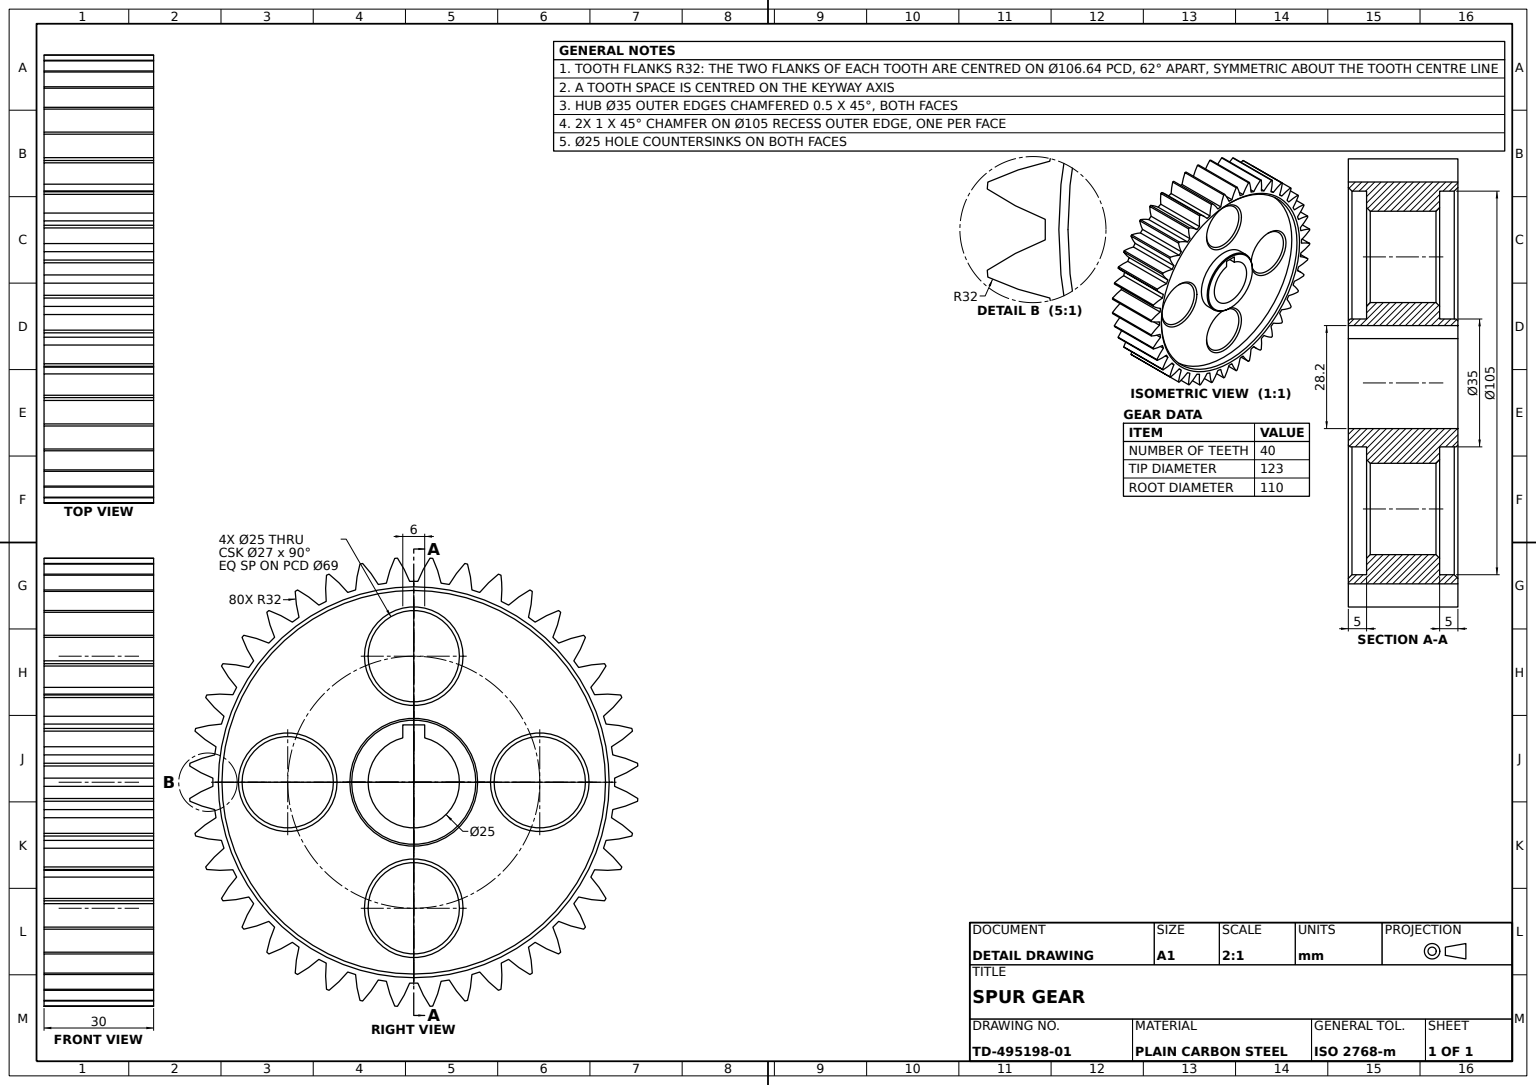
from build123d import *

# Parameters (mm, degrees)
GEAR_TOOTH_PROFILE_SKETCH_R       = 17.5
GEAR_BLANK_30MM_DEPTH             = 30
FRONT_RECESS_SKETCH_105_R         = 52.5
FRONT_WEB_RECESS_105X5_DEPTH      = 5
REAR_START                        = -5
REAR_RECESS_SKETCH_105_R          = 52.5
REAR_WEB_RECESS_105X5_DEPTH       = 5
REAR_RECESS_CHAMFER_1MM_SIZE      = 1
FRONT_RECESS_CHAMFER_1MM_SIZE     = 1
HUB_START                         = -20
HUB_SKETCH_35_R                   = 17.5
HUB_35_DEPTH                      = 20
KEYED_BORE_25_DEPTH               = 20
FRONT_START                       = 5
FRONT_HUB_BOSS_SKETCH_R           = 17.5
FRONT_HUB_BOSS_35X5_DEPTH         = 5
REAR_HUB_BOSS_SKETCH_R            = 17.5
REAR_HUB_BOSS_35X5_DEPTH          = 5
LIGHTENING_HOLES_SKETCH_4X_25_R   = 12.5
LIGHTENING_HOLES_4X_25_DEPTH      = 20
LIGHTENING_HOLE_CHAMFERS_1MM_SIZE = 1
FRONT_HUB_CHAMFER_0_5MM_SIZE      = 0.5
REAR_HUB_CHAMFER_0_5MM_SIZE       = 0.5


with BuildPart() as part:
    # Gear Tooth Profile Sketch → Gear Blank 30mm (new body)
    with BuildSketch(Plane.XY):
        with BuildLine():
            ThreePointArc((-13.990714351, 59.887477088), (-14.356889877, 59.800750104), (-14.722527887, 59.711784202))
            ThreePointArc((-14.722527887, 59.711784202), (-15.520987175, 56.212000648), (-15.922440287, 52.644808816))
            ThreePointArc((-15.922440287, 52.644808816), (-16.995934691, 52.308108396), (-18.062317448, 51.949520579))
            ThreePointArc((-18.062317448, 51.949520579), (-20.483842588, 54.599471175), (-23.186930882, 56.961532952))
            ThreePointArc((-23.186930882, 56.961532952), (-23.53503109, 56.818591249), (-23.882250156, 56.673522279))
            ThreePointArc((-23.882250156, 56.673522279), (-24.123392318, 53.091920316), (-23.961871129, 49.505845432))
            ThreePointArc((-23.961871129, 49.505845432), (-24.969477486, 49.00535883), (-25.966635809, 48.484366808))
            ThreePointArc((-25.966635809, 48.484366808), (-28.77289156, 50.722882124), (-31.812208221, 52.633006831))
            ThreePointArc((-31.812208221, 52.633006831), (-32.13366173, 52.437370108), (-32.453912166, 52.239770148))
            ThreePointArc((-32.453912166, 52.239770148), (-32.13179948, 48.664540704), (-31.41128118, 45.147883834))
            ThreePointArc((-31.41128118, 45.147883834), (-32.328188876, 44.495934691), (-33.231569417, 43.825367016))
            ThreePointArc((-33.231569417, 43.825367016), (-36.353456449, 45.597327377), (-39.654163416, 47.008481403))
            ThreePointArc((-39.654163416, 47.008481403), (-39.941054972, 46.764966884), (-40.22645115, 46.519701502))
            ThreePointArc((-40.22645115, 46.519701502), (-39.3490151, 43.038878591), (-38.08724124, 39.678231497))
            ThreePointArc((-38.08724124, 39.678231497), (-38.890872965, 38.890872965), (-39.678231497, 38.08724124))
            ThreePointArc((-39.678231497, 38.08724124), (-43.038878591, 39.3490151), (-46.519701502, 40.22645115))
            ThreePointArc((-46.519701502, 40.22645115), (-46.764966884, 39.941054972), (-47.008481403, 39.654163416))
            ThreePointArc((-47.008481403, 39.654163416), (-45.597327377, 36.353456449), (-43.825367016, 33.231569417))
            ThreePointArc((-43.825367016, 33.231569417), (-44.495934691, 32.328188876), (-45.147883834, 31.41128118))
            ThreePointArc((-45.147883834, 31.41128118), (-48.664540704, 32.13179948), (-52.239770148, 32.453912166))
            ThreePointArc((-52.239770148, 32.453912166), (-52.437370108, 32.13366173), (-52.633006831, 31.812208221))
            ThreePointArc((-52.633006831, 31.812208221), (-50.722882124, 28.77289156), (-48.484366808, 25.966635809))
            ThreePointArc((-48.484366808, 25.966635809), (-49.00535883, 24.969477486), (-49.505845432, 23.961871129))
            ThreePointArc((-49.505845432, 23.961871129), (-53.091920316, 24.123392318), (-56.673522279, 23.882250156))
            ThreePointArc((-56.673522279, 23.882250156), (-56.818591249, 23.53503109), (-56.961532952, 23.186930882))
            ThreePointArc((-56.961532952, 23.186930882), (-54.599471175, 20.483842588), (-51.949520579, 18.062317448))
            ThreePointArc((-51.949520579, 18.062317448), (-52.308108396, 16.995934691), (-52.644808816, 15.922440287))
            ThreePointArc((-52.644808816, 15.922440287), (-56.212000648, 15.520987175), (-59.711784202, 14.722527887))
            ThreePointArc((-59.711784202, 14.722527887), (-59.800750104, 14.356889877), (-59.887477088, 13.990714351))
            ThreePointArc((-59.887477088, 13.990714351), (-57.131640039, 11.690413431), (-54.135504743, 9.713244887))
            ThreePointArc((-54.135504743, 9.713244887), (-54.322858733, 8.603895577), (-54.487482289, 7.490946121))
            ThreePointArc((-54.487482289, 7.490946121), (-57.947954967, 6.536403817), (-61.279743827, 5.200288119))
            ThreePointArc((-61.279743827, 5.200288119), (-61.310416025, 4.825234387), (-61.338792782, 4.45))
            ThreePointArc((-61.338792782, 4.45), (-58.257038317, 2.609127496), (-54.988493114, 1.125))
            ThreePointArc((-54.988493114, 1.125), (-55, 0), (-54.988493114, -1.125))
            ThreePointArc((-54.988493114, -1.125), (-58.257038317, -2.609127496), (-61.338792782, -4.45))
            ThreePointArc((-61.338792782, -4.45), (-61.310416025, -4.825234387), (-61.279743827, -5.200288119))
            ThreePointArc((-61.279743827, -5.200288119), (-57.947954967, -6.536403817), (-54.487482289, -7.490946121))
            ThreePointArc((-54.487482289, -7.490946121), (-54.322858733, -8.603895577), (-54.135504743, -9.713244887))
            ThreePointArc((-54.135504743, -9.713244887), (-57.131640039, -11.690413431), (-59.887477088, -13.990714351))
            ThreePointArc((-59.887477088, -13.990714351), (-59.800750104, -14.356889877), (-59.711784202, -14.722527887))
            ThreePointArc((-59.711784202, -14.722527887), (-56.212000648, -15.520987175), (-52.644808816, -15.922440287))
            ThreePointArc((-52.644808816, -15.922440287), (-52.308108396, -16.995934691), (-51.949520579, -18.062317448))
            ThreePointArc((-51.949520579, -18.062317448), (-54.599471175, -20.483842588), (-56.961532952, -23.186930882))
            ThreePointArc((-56.961532952, -23.186930882), (-56.818591249, -23.53503109), (-56.673522279, -23.882250156))
            ThreePointArc((-56.673522279, -23.882250156), (-53.091920316, -24.123392318), (-49.505845432, -23.961871129))
            ThreePointArc((-49.505845432, -23.961871129), (-49.00535883, -24.969477486), (-48.484366808, -25.966635809))
            ThreePointArc((-48.484366808, -25.966635809), (-50.722882124, -28.77289156), (-52.633006831, -31.812208221))
            ThreePointArc((-52.633006831, -31.812208221), (-52.437370108, -32.13366173), (-52.239770148, -32.453912166))
            ThreePointArc((-52.239770148, -32.453912166), (-48.664540704, -32.13179948), (-45.147883834, -31.41128118))
            ThreePointArc((-45.147883834, -31.41128118), (-44.495934691, -32.328188876), (-43.825367016, -33.231569417))
            ThreePointArc((-43.825367016, -33.231569417), (-45.597327377, -36.353456449), (-47.008481403, -39.654163416))
            ThreePointArc((-47.008481403, -39.654163416), (-46.764966884, -39.941054972), (-46.519701502, -40.22645115))
            ThreePointArc((-46.519701502, -40.22645115), (-43.038878591, -39.3490151), (-39.678231497, -38.08724124))
            ThreePointArc((-39.678231497, -38.08724124), (-38.890872965, -38.890872965), (-38.08724124, -39.678231497))
            ThreePointArc((-38.08724124, -39.678231497), (-39.3490151, -43.038878591), (-40.22645115, -46.519701502))
            ThreePointArc((-40.22645115, -46.519701502), (-39.941054972, -46.764966884), (-39.654163416, -47.008481403))
            ThreePointArc((-39.654163416, -47.008481403), (-36.353456449, -45.597327377), (-33.231569417, -43.825367016))
            ThreePointArc((-33.231569417, -43.825367016), (-32.328188876, -44.495934691), (-31.41128118, -45.147883834))
            ThreePointArc((-31.41128118, -45.147883834), (-32.13179948, -48.664540704), (-32.453912166, -52.239770148))
            ThreePointArc((-32.453912166, -52.239770148), (-32.13366173, -52.437370108), (-31.812208221, -52.633006831))
            ThreePointArc((-31.812208221, -52.633006831), (-28.77289156, -50.722882124), (-25.966635809, -48.484366808))
            ThreePointArc((-25.966635809, -48.484366808), (-24.969477486, -49.00535883), (-23.961871129, -49.505845432))
            ThreePointArc((-23.961871129, -49.505845432), (-24.123392318, -53.091920316), (-23.882250156, -56.673522279))
            ThreePointArc((-23.882250156, -56.673522279), (-23.53503109, -56.818591249), (-23.186930882, -56.961532952))
            ThreePointArc((-23.186930882, -56.961532952), (-20.483842588, -54.599471175), (-18.062317448, -51.949520579))
            ThreePointArc((-18.062317448, -51.949520579), (-16.995934691, -52.308108396), (-15.922440287, -52.644808816))
            ThreePointArc((-15.922440287, -52.644808816), (-15.520987175, -56.212000648), (-14.722527887, -59.711784202))
            ThreePointArc((-14.722527887, -59.711784202), (-14.356889877, -59.800750104), (-13.990714351, -59.887477088))
            ThreePointArc((-13.990714351, -59.887477088), (-11.690413431, -57.131640039), (-9.713244887, -54.135504743))
            ThreePointArc((-9.713244887, -54.135504743), (-8.603895577, -54.322858733), (-7.490946121, -54.487482289))
            ThreePointArc((-7.490946121, -54.487482289), (-6.536403817, -57.947954967), (-5.200288119, -61.279743827))
            ThreePointArc((-5.200288119, -61.279743827), (-4.825234387, -61.310416025), (-4.45, -61.338792782))
            ThreePointArc((-4.45, -61.338792782), (-2.609127496, -58.257038317), (-1.125, -54.988493114))
            ThreePointArc((-1.125, -54.988493114), (0, -55), (1.125, -54.988493114))
            ThreePointArc((1.125, -54.988493114), (2.609127496, -58.257038317), (4.45, -61.338792782))
            ThreePointArc((4.45, -61.338792782), (4.825234387, -61.310416025), (5.200288119, -61.279743827))
            ThreePointArc((5.200288119, -61.279743827), (6.536403817, -57.947954967), (7.490946121, -54.487482289))
            ThreePointArc((7.490946121, -54.487482289), (8.603895577, -54.322858733), (9.713244887, -54.135504743))
            ThreePointArc((9.713244887, -54.135504743), (11.690413431, -57.131640039), (13.990714351, -59.887477088))
            ThreePointArc((13.990714351, -59.887477088), (14.356889877, -59.800750104), (14.722527887, -59.711784202))
            ThreePointArc((14.722527887, -59.711784202), (15.520987175, -56.212000648), (15.922440287, -52.644808816))
            ThreePointArc((15.922440287, -52.644808816), (16.995934691, -52.308108396), (18.062317448, -51.949520579))
            ThreePointArc((18.062317448, -51.949520579), (20.483842588, -54.599471175), (23.186930882, -56.961532952))
            ThreePointArc((23.186930882, -56.961532952), (23.53503109, -56.818591249), (23.882250156, -56.673522279))
            ThreePointArc((23.882250156, -56.673522279), (24.123392318, -53.091920316), (23.961871129, -49.505845432))
            ThreePointArc((23.961871129, -49.505845432), (24.969477486, -49.00535883), (25.966635809, -48.484366808))
            ThreePointArc((25.966635809, -48.484366808), (28.77289156, -50.722882124), (31.812208221, -52.633006831))
            ThreePointArc((31.812208221, -52.633006831), (32.13366173, -52.437370108), (32.453912166, -52.239770148))
            ThreePointArc((32.453912166, -52.239770148), (32.13179948, -48.664540704), (31.41128118, -45.147883834))
            ThreePointArc((31.41128118, -45.147883834), (32.328188876, -44.495934691), (33.231569417, -43.825367016))
            ThreePointArc((33.231569417, -43.825367016), (36.353456449, -45.597327377), (39.654163416, -47.008481403))
            ThreePointArc((39.654163416, -47.008481403), (39.941054972, -46.764966884), (40.22645115, -46.519701502))
            ThreePointArc((40.22645115, -46.519701502), (39.3490151, -43.038878591), (38.08724124, -39.678231497))
            ThreePointArc((38.08724124, -39.678231497), (38.890872965, -38.890872965), (39.678231497, -38.08724124))
            ThreePointArc((39.678231497, -38.08724124), (43.038878591, -39.3490151), (46.519701502, -40.22645115))
            ThreePointArc((46.519701502, -40.22645115), (46.764966884, -39.941054972), (47.008481403, -39.654163416))
            ThreePointArc((47.008481403, -39.654163416), (45.597327377, -36.353456449), (43.825367016, -33.231569417))
            ThreePointArc((43.825367016, -33.231569417), (44.495934691, -32.328188876), (45.147883834, -31.41128118))
            ThreePointArc((45.147883834, -31.41128118), (48.664540704, -32.13179948), (52.239770148, -32.453912166))
            ThreePointArc((52.239770148, -32.453912166), (52.437370108, -32.13366173), (52.633006831, -31.812208221))
            ThreePointArc((52.633006831, -31.812208221), (50.722882124, -28.77289156), (48.484366808, -25.966635809))
            ThreePointArc((48.484366808, -25.966635809), (49.00535883, -24.969477486), (49.505845432, -23.961871129))
            ThreePointArc((49.505845432, -23.961871129), (53.091920316, -24.123392318), (56.673522279, -23.882250156))
            ThreePointArc((56.673522279, -23.882250156), (56.818591249, -23.53503109), (56.961532952, -23.186930882))
            ThreePointArc((56.961532952, -23.186930882), (54.599471175, -20.483842588), (51.949520579, -18.062317448))
            ThreePointArc((51.949520579, -18.062317448), (52.308108396, -16.995934691), (52.644808816, -15.922440287))
            ThreePointArc((52.644808816, -15.922440287), (56.212000648, -15.520987175), (59.711784202, -14.722527887))
            ThreePointArc((59.711784202, -14.722527887), (59.800750104, -14.356889877), (59.887477088, -13.990714351))
            ThreePointArc((59.887477088, -13.990714351), (57.131640039, -11.690413431), (54.135504743, -9.713244887))
            ThreePointArc((54.135504743, -9.713244887), (54.322858733, -8.603895577), (54.487482289, -7.490946121))
            ThreePointArc((54.487482289, -7.490946121), (57.947954967, -6.536403817), (61.279743827, -5.200288119))
            ThreePointArc((61.279743827, -5.200288119), (61.310416025, -4.825234387), (61.338792782, -4.45))
            ThreePointArc((61.338792782, -4.45), (58.257038317, -2.609127496), (54.988493114, -1.125))
            ThreePointArc((54.988493114, -1.125), (55, 0), (54.988493114, 1.125))
            ThreePointArc((54.988493114, 1.125), (58.257038317, 2.609127496), (61.338792782, 4.45))
            ThreePointArc((61.338792782, 4.45), (61.310416025, 4.825234387), (61.279743827, 5.200288119))
            ThreePointArc((61.279743827, 5.200288119), (57.947954967, 6.536403817), (54.487482289, 7.490946121))
            ThreePointArc((54.487482289, 7.490946121), (54.322858733, 8.603895577), (54.135504743, 9.713244887))
            ThreePointArc((54.135504743, 9.713244887), (57.131640039, 11.690413431), (59.887477088, 13.990714351))
            ThreePointArc((59.887477088, 13.990714351), (59.800750104, 14.356889877), (59.711784202, 14.722527887))
            ThreePointArc((59.711784202, 14.722527887), (56.212000648, 15.520987175), (52.644808816, 15.922440287))
            ThreePointArc((52.644808816, 15.922440287), (52.308108396, 16.995934691), (51.949520579, 18.062317448))
            ThreePointArc((51.949520579, 18.062317448), (54.599471175, 20.483842588), (56.961532952, 23.186930882))
            ThreePointArc((56.961532952, 23.186930882), (56.818591249, 23.53503109), (56.673522279, 23.882250156))
            ThreePointArc((56.673522279, 23.882250156), (53.091920316, 24.123392318), (49.505845432, 23.961871129))
            ThreePointArc((49.505845432, 23.961871129), (49.00535883, 24.969477486), (48.484366808, 25.966635809))
            ThreePointArc((48.484366808, 25.966635809), (50.722882124, 28.77289156), (52.633006831, 31.812208221))
            ThreePointArc((52.633006831, 31.812208221), (52.437370108, 32.13366173), (52.239770148, 32.453912166))
            ThreePointArc((52.239770148, 32.453912166), (48.664540704, 32.13179948), (45.147883834, 31.41128118))
            ThreePointArc((45.147883834, 31.41128118), (44.495934691, 32.328188876), (43.825367016, 33.231569417))
            ThreePointArc((43.825367016, 33.231569417), (45.597327377, 36.353456449), (47.008481403, 39.654163416))
            ThreePointArc((47.008481403, 39.654163416), (46.764966884, 39.941054972), (46.519701502, 40.22645115))
            ThreePointArc((46.519701502, 40.22645115), (43.038878591, 39.3490151), (39.678231497, 38.08724124))
            ThreePointArc((39.678231497, 38.08724124), (38.890872965, 38.890872965), (38.08724124, 39.678231497))
            ThreePointArc((38.08724124, 39.678231497), (39.3490151, 43.038878591), (40.22645115, 46.519701502))
            ThreePointArc((40.22645115, 46.519701502), (39.941054972, 46.764966884), (39.654163416, 47.008481403))
            ThreePointArc((39.654163416, 47.008481403), (36.353456449, 45.597327377), (33.231569417, 43.825367016))
            ThreePointArc((33.231569417, 43.825367016), (32.328188876, 44.495934691), (31.41128118, 45.147883834))
            ThreePointArc((31.41128118, 45.147883834), (32.13179948, 48.664540704), (32.453912166, 52.239770148))
            ThreePointArc((32.453912166, 52.239770148), (32.13366173, 52.437370108), (31.812208221, 52.633006831))
            ThreePointArc((31.812208221, 52.633006831), (28.77289156, 50.722882124), (25.966635809, 48.484366808))
            ThreePointArc((25.966635809, 48.484366808), (24.969477486, 49.00535883), (23.961871129, 49.505845432))
            ThreePointArc((23.961871129, 49.505845432), (24.123392318, 53.091920316), (23.882250156, 56.673522279))
            ThreePointArc((23.882250156, 56.673522279), (23.53503109, 56.818591249), (23.186930882, 56.961532952))
            ThreePointArc((23.186930882, 56.961532952), (20.483842588, 54.599471175), (18.062317448, 51.949520579))
            ThreePointArc((18.062317448, 51.949520579), (16.995934691, 52.308108396), (15.922440287, 52.644808816))
            ThreePointArc((15.922440287, 52.644808816), (15.520987175, 56.212000648), (14.722527887, 59.711784202))
            ThreePointArc((14.722527887, 59.711784202), (14.356889877, 59.800750104), (13.990714351, 59.887477088))
            ThreePointArc((13.990714351, 59.887477088), (11.690413431, 57.131640039), (9.713244887, 54.135504743))
            ThreePointArc((9.713244887, 54.135504743), (8.603895577, 54.322858733), (7.490946121, 54.487482289))
            ThreePointArc((7.490946121, 54.487482289), (6.536403817, 57.947954967), (5.200288119, 61.279743827))
            ThreePointArc((5.200288119, 61.279743827), (4.825234387, 61.310416025), (4.45, 61.338792782))
            ThreePointArc((4.45, 61.338792782), (2.609127496, 58.257038317), (1.125, 54.988493114))
            ThreePointArc((1.125, 54.988493114), (0, 55), (-1.125, 54.988493114))
            ThreePointArc((-1.125, 54.988493114), (-2.609127496, 58.257038317), (-4.45, 61.338792782))
            ThreePointArc((-4.45, 61.338792782), (-4.825234387, 61.310416025), (-5.200288119, 61.279743827))
            ThreePointArc((-5.200288119, 61.279743827), (-6.536403817, 57.947954967), (-7.490946121, 54.487482289))
            ThreePointArc((-7.490946121, 54.487482289), (-8.603895577, 54.322858733), (-9.713244887, 54.135504743))
            ThreePointArc((-9.713244887, 54.135504743), (-11.690413431, 57.131640039), (-13.990714351, 59.887477088))
        make_face()
        Circle(GEAR_TOOTH_PROFILE_SKETCH_R, mode=Mode.SUBTRACT)
    extrude(amount=GEAR_BLANK_30MM_DEPTH)

    # Front Recess Sketch Ø105 → Front Web Recess Ø105x5 (cut)
    with BuildSketch(Plane.XY.offset(30)):
        Circle(FRONT_RECESS_SKETCH_105_R)
    extrude(amount=-FRONT_WEB_RECESS_105X5_DEPTH, mode=Mode.SUBTRACT)

    # Rear Recess Sketch Ø105 → Rear Web Recess Ø105x5 (cut)
    with BuildSketch(Plane(origin=(0, 0, 0), x_dir=(-1, 0, 0), z_dir=(0, 0, -1)).offset(REAR_START)):
        with Locations(Location((0, 0, 0), (0, 0, 180))):
            Circle(REAR_RECESS_SKETCH_105_R)
    extrude(amount=REAR_WEB_RECESS_105X5_DEPTH, mode=Mode.SUBTRACT)

    # Rear Recess Chamfer 1mm
    rear_recess_chamfer_1mm_edges = [part.edges().sort_by_distance(p)[0] for p in [
        (-52.5, 0, 0),
    ]]
    chamfer(rear_recess_chamfer_1mm_edges, length=REAR_RECESS_CHAMFER_1MM_SIZE)

    # Front Recess Chamfer 1mm
    front_recess_chamfer_1mm_edges = [part.edges().sort_by_distance(p)[0] for p in [
        (-52.5, 0, 30),
    ]]
    chamfer(front_recess_chamfer_1mm_edges, length=FRONT_RECESS_CHAMFER_1MM_SIZE)

    # Hub Sketch Ø35 → Hub Ø35 (add)
    with BuildSketch(Plane.XY.offset(25).offset(HUB_START)):
        Circle(HUB_SKETCH_35_R)
    extrude(amount=HUB_35_DEPTH)

    # Keyed Bore Sketch → Keyed Bore Ø25 (cut)
    with BuildSketch(Plane.XY.offset(25)):
        with BuildLine():
            Line((3, 12.1346611), (3, 15.7))
            Line((3, 15.7), (-3, 15.7))
            Line((-3, 15.7), (-3, 12.1346611))
            ThreePointArc((-3, 12.1346611), (0, -12.5), (3, 12.1346611))
        make_face()
    extrude(amount=-KEYED_BORE_25_DEPTH, mode=Mode.SUBTRACT)

    # Front Hub Boss Sketch → Front Hub Boss Ø35x5 (add)
    with BuildSketch(Plane.XY.offset(25).offset(FRONT_START)):
        Circle(FRONT_HUB_BOSS_SKETCH_R)
        with BuildLine():
            Line((-3, 12.1346611), (-3, 15.7))
            Line((-3, 15.7), (3, 15.7))
            Line((3, 15.7), (3, 12.1346611))
            ThreePointArc((3, 12.1346611), (0, -12.5), (-3, 12.1346611))
        make_face(mode=Mode.SUBTRACT)
    extrude(amount=-FRONT_HUB_BOSS_35X5_DEPTH)

    # Rear Hub Boss Sketch → Rear Hub Boss Ø35x5 (add)
    with BuildSketch(Plane(origin=(0, 0, 5), x_dir=(-1, 0, 0), z_dir=(0, 0, -1))):
        with Locations(Location((0, 0, 0), (0, 0, 180))):
            Circle(REAR_HUB_BOSS_SKETCH_R)
        with BuildLine():
            Line((-3, 12.1346611), (-3, 15.7))
            Line((-3, 15.7), (3, 15.7))
            Line((3, 15.7), (3, 12.1346611))
            ThreePointArc((3, 12.1346611), (0, -12.5), (-3, 12.1346611))
        make_face(mode=Mode.SUBTRACT)
    extrude(amount=REAR_HUB_BOSS_35X5_DEPTH)

    # Lightening Holes Sketch 4xØ25 → Lightening Holes 4xØ25 (cut)
    with BuildSketch(Plane.XY.offset(25)):
        with Locations((0, 34.5)):
            Circle(LIGHTENING_HOLES_SKETCH_4X_25_R)
        with Locations((34.5, 0)):
            Circle(LIGHTENING_HOLES_SKETCH_4X_25_R)
        with Locations((0, -34.5)):
            Circle(LIGHTENING_HOLES_SKETCH_4X_25_R)
        with Locations((-34.5, 0)):
            Circle(LIGHTENING_HOLES_SKETCH_4X_25_R)
    extrude(amount=-LIGHTENING_HOLES_4X_25_DEPTH, mode=Mode.SUBTRACT)

    # Lightening Hole Chamfers 1mm
    lightening_hole_chamfers_1mm_edges = [part.edges().sort_by_distance(p)[0] for p in [
        (-12.5, 34.5, 5),
        (-12.5, 34.5, 25),
        (22, 0, 5),
        (22, 0, 25),
        (-12.5, -34.5, 5),
        (-12.5, -34.5, 25),
        (-47, 0, 5),
        (-47, 0, 25),
    ]]
    chamfer(lightening_hole_chamfers_1mm_edges, length=LIGHTENING_HOLE_CHAMFERS_1MM_SIZE)

    # Front Hub Chamfer 0.5mm
    front_hub_chamfer_0_5mm_edges = [part.edges().sort_by_distance(p)[0] for p in [
        (-17.5, 0, 30),
    ]]
    chamfer(front_hub_chamfer_0_5mm_edges, length=FRONT_HUB_CHAMFER_0_5MM_SIZE)

    # Rear Hub Chamfer 0.5mm
    rear_hub_chamfer_0_5mm_edges = [part.edges().sort_by_distance(p)[0] for p in [
        (-17.5, 0, 0),
    ]]
    chamfer(rear_hub_chamfer_0_5mm_edges, length=REAR_HUB_CHAMFER_0_5MM_SIZE)


solid = part.part
